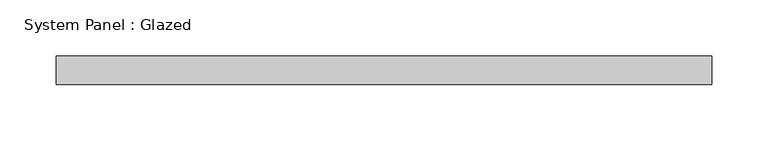
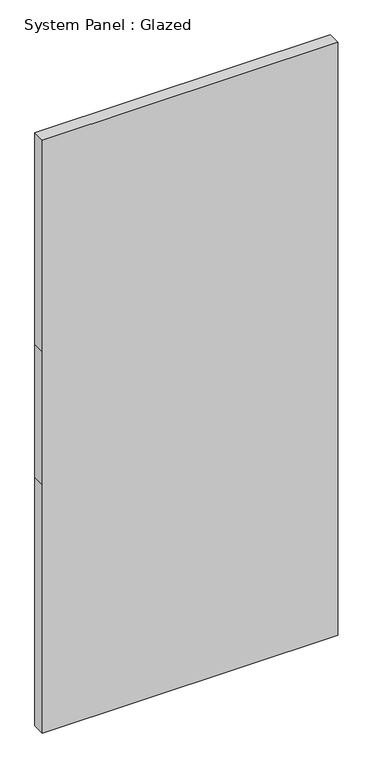
"""IFC4 building model written with IfcOpenShell, lengths in millimetres: plate geometry, System Panel : Glazed."""

from ifc_helpers import new_model, si_unit, frame, origin, place, context, project, spatial, polyline, outline, extrude, source, transform, mapped, element, save


def system_panel_glazed_fe088b68(model_context):
    return source(origin(), model_context, "Body", "SweptSolid", [
        extrude(outline(polyline([(0.0, -292.1), (0.0, 292.1), (519.0903046, 292.1), (797.6854569, 292.1), (1239.7709137, 292.1), (1239.7709137, -292.1), (797.6854569, -292.1), (519.0903046, -292.1), (0.0, -292.1)])), frame((0.0, 19.05, 0.0), z_axis=(0.0, 1.0, 0.0), x_axis=(0.0, 0.0, 1.0)), (0.0, 0.0, 1.0), 25.4),
    ])


if __name__ == "__main__":
    model = new_model("IFC4")
    model_context = context("Model", 3, world=origin())
    ifc_project = project(units=[si_unit("LENGTHUNIT", "METRE", prefix="MILLI")], contexts=[model_context])
    site = spatial("IfcSite", under=ifc_project)
    building = spatial("IfcBuilding", under=site)
    placement = place(None, origin())
    system_panel_glazed_shape = system_panel_glazed_fe088b68(model_context)
    element("IfcPlate", 1, ObjectType="System Panel : Glazed", at=placement, inside=building, context=model_context, shape_type="MappedRepresentation", body=[
        mapped(system_panel_glazed_shape, transform((0.0, 0.0, 0.0), x_axis=(1.0, 0.0, 0.0), y_axis=(0.0, 1.0, 0.0), z_axis=(0.0, 0.0, 1.0))),
    ])
    save(model, "model.ifc")

# Revit data of these elements
# Type "System Panel : Glazed"
#   Construction Type Id = "GSP4R"
#   Analytic Construction = "1/8 in Pilkington single glazing"
#   Visual Light Transmittance = 0.9
#   Solar Heat Gain Coefficient = 0.86
#   Heat Transfer Coefficient (U) = 1.18115 BTU/(h·ft²·°F)
#   Define Thermal Properties by = 1
# Element 1 (IfcPlate, "System Panel : Glazed")
#   Materials on its faces: "Glass"
# Materials
#   "Glass": class "Glass", colour RGB 0 128 192, transparency 0.75, Description = "Soda Lime Glass", Cost = 0
